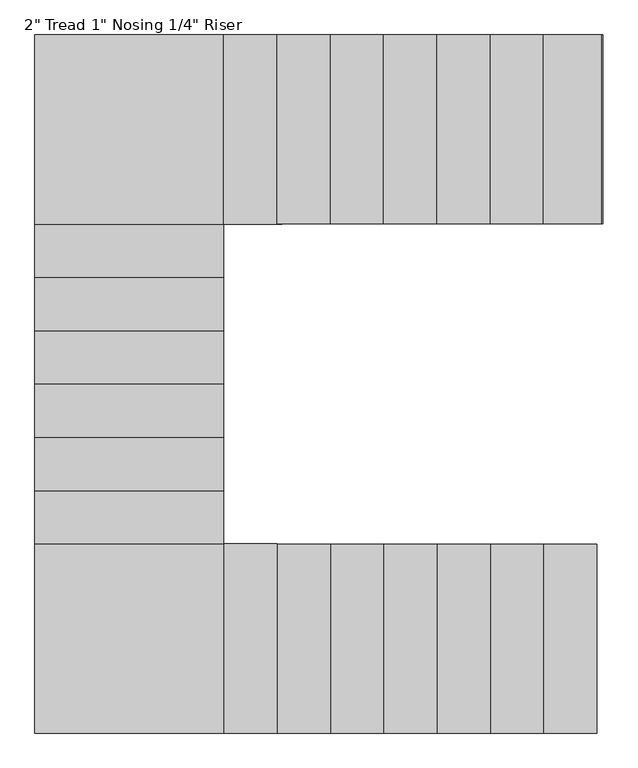
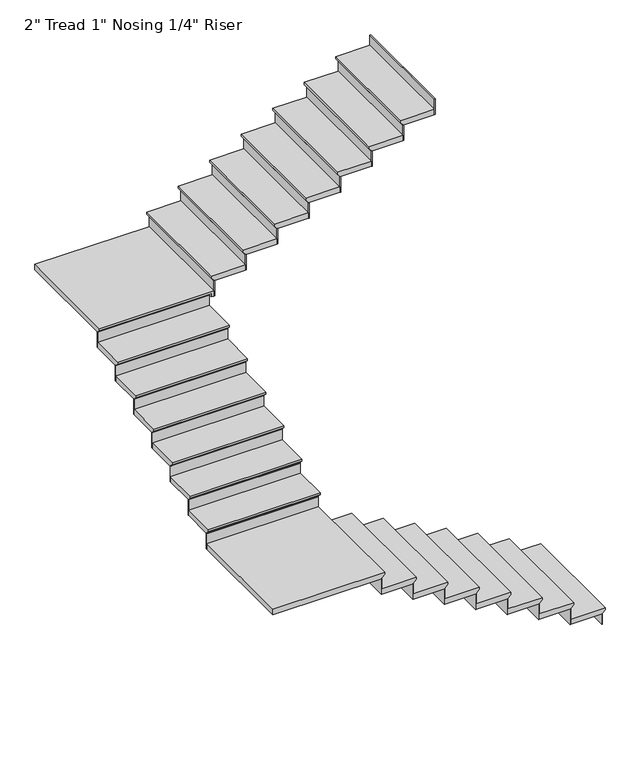
"""IFC4 building model written with IfcOpenShell, lengths in millimetres: stair flight geometry."""

from ifc_helpers import new_model, si_unit, origin, place, context, project, spatial, faceted_brep, source, transform, mapped, element, save


def stair_flight_cb67390f(model_context):
    return source(origin(), model_context, "Body", "Brep", [
        faceted_brep([(14750.242447, -127.8399287, 126.0928571), (14750.242447, -127.8399287, 145.1428571), (14750.242447, -1118.4399287, 145.1428571), (14750.242447, -1118.4399287, 126.0928571), (14724.842447, -127.8399287, 100.6928571), (14724.842447, -1118.4399287, 100.6928571), (14445.442447, -127.8399287, 145.1428571), (14445.442447, -1118.4399287, 145.1428571), (14724.842447, -1118.4399287, 94.3428571), (14445.442447, -1118.4399287, 94.3428571), (14445.442447, -127.8399287, 94.3428571), (14724.842447, -127.8399287, 94.3428571)], [[[0, 1, 2, 3]], [[4, 0, 3, 5]], [[2, 1, 6, 7]], [[8, 9, 10, 11]], [[2, 7, 9, 8, 5, 3]], [[8, 11, 4, 5]], [[6, 1, 0, 4, 11, 10]], [[7, 6, 10, 9]]]),
        faceted_brep([(14724.842447, -127.8399287, 94.3428571), (14724.842447, -127.8399287, 0.0), (14718.492447, -127.8399287, 0.0), (14718.492447, -127.8399287, 94.3428571), (14724.842447, -1118.4399287, 94.3428571), (14718.492447, -1118.4399287, 94.3428571), (14718.492447, -1118.4399287, 0.0), (14724.842447, -1118.4399287, 0.0)], [[[0, 1, 2, 3]], [[4, 5, 6, 7]], [[1, 0, 4, 7]], [[2, 1, 7, 6]], [[3, 2, 6, 5]], [[0, 3, 5, 4]]]),
        faceted_brep([(14445.442447, -127.8399287, 239.4857143), (14445.442447, -127.8399287, 94.3428571), (14439.092447, -127.8399287, 94.3428571), (14439.092447, -127.8399287, 239.4857143), (14445.442447, -1118.4399287, 239.4857143), (14439.092447, -1118.4399287, 239.4857143), (14439.092447, -1118.4399287, 94.3428571), (14445.442447, -1118.4399287, 94.3428571)], [[[0, 1, 2, 3]], [[4, 5, 6, 7]], [[1, 0, 4, 7]], [[2, 1, 7, 6]], [[3, 2, 6, 5]], [[0, 3, 5, 4]]]),
        faceted_brep([(14470.842447, -1118.4399287, 290.2857143), (14470.842447, -127.8399287, 290.2857143), (14166.042447, -127.8399287, 290.2857143), (14166.042447, -1118.4399287, 290.2857143), (14445.442447, -1118.4399287, 239.4857143), (14166.042447, -1118.4399287, 239.4857143), (14166.042447, -127.8399287, 239.4857143), (14445.442447, -127.8399287, 239.4857143), (14445.442447, -1118.4399287, 245.8357143), (14470.842447, -1118.4399287, 271.2357143), (14445.442447, -127.8399287, 245.8357143), (14470.842447, -127.8399287, 271.2357143)], [[[0, 1, 2, 3]], [[4, 5, 6, 7]], [[0, 3, 5, 4, 8, 9]], [[4, 7, 10, 8]], [[2, 1, 11, 10, 7, 6]], [[3, 2, 6, 5]], [[11, 1, 0, 9]], [[10, 11, 9, 8]]]),
        faceted_brep([(14166.042447, -127.8399287, 384.6285714), (14166.042447, -127.8399287, 239.4857143), (14159.692447, -127.8399287, 239.4857143), (14159.692447, -127.8399287, 384.6285714), (14166.042447, -1118.4399287, 384.6285714), (14159.692447, -1118.4399287, 384.6285714), (14159.692447, -1118.4399287, 239.4857143), (14166.042447, -1118.4399287, 239.4857143)], [[[0, 1, 2, 3]], [[4, 5, 6, 7]], [[1, 0, 4, 7]], [[2, 1, 7, 6]], [[3, 2, 6, 5]], [[0, 3, 5, 4]]]),
        faceted_brep([(14191.442447, -1118.4399287, 435.4285714), (14191.442447, -127.8399287, 435.4285714), (13886.642447, -127.8399287, 435.4285714), (13886.642447, -1118.4399287, 435.4285714), (14166.042447, -1118.4399287, 384.6285714), (13886.642447, -1118.4399287, 384.6285714), (13886.642447, -127.8399287, 384.6285714), (14166.042447, -127.8399287, 384.6285714), (14166.042447, -1118.4399287, 390.9785714), (14191.442447, -1118.4399287, 416.3785714), (14166.042447, -127.8399287, 390.9785714), (14191.442447, -127.8399287, 416.3785714)], [[[0, 1, 2, 3]], [[4, 5, 6, 7]], [[0, 3, 5, 4, 8, 9]], [[4, 7, 10, 8]], [[2, 1, 11, 10, 7, 6]], [[3, 2, 6, 5]], [[11, 1, 0, 9]], [[10, 11, 9, 8]]]),
        faceted_brep([(13886.642447, -127.8399287, 529.7714286), (13886.642447, -127.8399287, 384.6285714), (13880.292447, -127.8399287, 384.6285714), (13880.292447, -127.8399287, 529.7714286), (13886.642447, -1118.4399287, 529.7714286), (13880.292447, -1118.4399287, 529.7714286), (13880.292447, -1118.4399287, 384.6285714), (13886.642447, -1118.4399287, 384.6285714)], [[[0, 1, 2, 3]], [[4, 5, 6, 7]], [[1, 0, 4, 7]], [[2, 1, 7, 6]], [[3, 2, 6, 5]], [[0, 3, 5, 4]]]),
        faceted_brep([(13912.042447, -1118.4399287, 580.5714286), (13912.042447, -127.8399287, 580.5714286), (13607.242447, -127.8399287, 580.5714286), (13607.242447, -1118.4399287, 580.5714286), (13886.642447, -1118.4399287, 529.7714286), (13607.242447, -1118.4399287, 529.7714286), (13607.242447, -127.8399287, 529.7714286), (13886.642447, -127.8399287, 529.7714286), (13886.642447, -1118.4399287, 536.1214286), (13912.042447, -1118.4399287, 561.5214286), (13886.642447, -127.8399287, 536.1214286), (13912.042447, -127.8399287, 561.5214286)], [[[0, 1, 2, 3]], [[4, 5, 6, 7]], [[0, 3, 5, 4, 8, 9]], [[4, 7, 10, 8]], [[2, 1, 11, 10, 7, 6]], [[3, 2, 6, 5]], [[11, 1, 0, 9]], [[10, 11, 9, 8]]]),
        faceted_brep([(13607.242447, -127.8399287, 674.9142857), (13607.242447, -127.8399287, 529.7714286), (13600.892447, -127.8399287, 529.7714286), (13600.892447, -127.8399287, 674.9142857), (13607.242447, -1118.4399287, 674.9142857), (13600.892447, -1118.4399287, 674.9142857), (13600.892447, -1118.4399287, 529.7714286), (13607.242447, -1118.4399287, 529.7714286)], [[[0, 1, 2, 3]], [[4, 5, 6, 7]], [[1, 0, 4, 7]], [[2, 1, 7, 6]], [[3, 2, 6, 5]], [[0, 3, 5, 4]]]),
        faceted_brep([(13632.642447, -1118.4399287, 725.7142857), (13632.642447, -127.8399287, 725.7142857), (13327.842447, -127.8399287, 725.7142857), (13327.842447, -1118.4399287, 725.7142857), (13607.242447, -1118.4399287, 674.9142857), (13327.842447, -1118.4399287, 674.9142857), (13327.842447, -127.8399287, 674.9142857), (13607.242447, -127.8399287, 674.9142857), (13607.242447, -1118.4399287, 681.2642857), (13632.642447, -1118.4399287, 706.6642857), (13607.242447, -127.8399287, 681.2642857), (13632.642447, -127.8399287, 706.6642857)], [[[0, 1, 2, 3]], [[4, 5, 6, 7]], [[0, 3, 5, 4, 8, 9]], [[4, 7, 10, 8]], [[2, 1, 11, 10, 7, 6]], [[3, 2, 6, 5]], [[11, 1, 0, 9]], [[10, 11, 9, 8]]]),
        faceted_brep([(13327.842447, -127.8399287, 820.0571429), (13327.842447, -127.8399287, 674.9142857), (13321.492447, -127.8399287, 674.9142857), (13321.492447, -127.8399287, 820.0571429), (13327.842447, -1118.4399287, 820.0571429), (13321.492447, -1118.4399287, 820.0571429), (13321.492447, -1118.4399287, 674.9142857), (13327.842447, -1118.4399287, 674.9142857)], [[[0, 1, 2, 3]], [[4, 5, 6, 7]], [[1, 0, 4, 7]], [[2, 1, 7, 6]], [[3, 2, 6, 5]], [[0, 3, 5, 4]]]),
        faceted_brep([(13353.242447, -1118.4399287, 870.8571429), (13353.242447, -127.8399287, 870.8571429), (13048.442447, -127.8399287, 870.8571429), (13048.442447, -1118.4399287, 870.8571429), (13327.842447, -1118.4399287, 820.0571429), (13048.442447, -1118.4399287, 820.0571429), (13048.442447, -127.8399287, 820.0571429), (13327.842447, -127.8399287, 820.0571429), (13327.842447, -1118.4399287, 826.4071429), (13353.242447, -1118.4399287, 851.8071429), (13327.842447, -127.8399287, 826.4071429), (13353.242447, -127.8399287, 851.8071429)], [[[0, 1, 2, 3]], [[4, 5, 6, 7]], [[0, 3, 5, 4, 8, 9]], [[4, 7, 10, 8]], [[2, 1, 11, 10, 7, 6]], [[3, 2, 6, 5]], [[11, 1, 0, 9]], [[10, 11, 9, 8]]]),
        faceted_brep([(13048.442447, -127.8399287, 965.2), (13048.442447, -127.8399287, 820.0571429), (13042.092447, -127.8399287, 820.0571429), (13042.092447, -127.8399287, 965.2), (13048.442447, -1118.4399287, 965.2), (13042.092447, -1118.4399287, 965.2), (13042.092447, -1118.4399287, 820.0571429), (13048.442447, -1118.4399287, 820.0571429)], [[[0, 1, 2, 3]], [[4, 5, 6, 7]], [[1, 0, 4, 7]], [[2, 1, 7, 6]], [[3, 2, 6, 5]], [[0, 3, 5, 4]]]),
        faceted_brep([(13073.842447, -1118.4399287, 1016.0), (13073.842447, -127.8399287, 1016.0), (12769.042447, -127.8399287, 1016.0), (12769.042447, -1118.4399287, 1016.0), (13048.442447, -1118.4399287, 965.2), (12769.042447, -1118.4399287, 965.2), (12769.042447, -127.8399287, 965.2), (13048.442447, -127.8399287, 965.2), (13048.442447, -1118.4399287, 971.55), (13073.842447, -1118.4399287, 996.95), (13048.442447, -127.8399287, 971.55), (13073.842447, -127.8399287, 996.95)], [[[0, 1, 2, 3]], [[4, 5, 6, 7]], [[0, 3, 5, 4, 8, 9]], [[4, 7, 10, 8]], [[2, 1, 11, 10, 7, 6]], [[3, 2, 6, 5]], [[11, 1, 0, 9]], [[10, 11, 9, 8]]]),
        faceted_brep([(12769.042447, -127.8399287, 1110.3428571), (12769.042447, -127.8399287, 965.2), (12762.692447, -127.8399287, 965.2), (12762.692447, -127.8399287, 1110.3428571), (12769.042447, -1118.4399287, 1110.3428571), (12762.692447, -1118.4399287, 1110.3428571), (12762.692447, -1118.4399287, 965.2), (12769.042447, -1118.4399287, 965.2)], [[[0, 1, 2, 3]], [[4, 5, 6, 7]], [[1, 0, 4, 7]], [[2, 1, 7, 6]], [[3, 2, 6, 5]], [[0, 3, 5, 4]]]),
        faceted_brep([(11803.842447, -102.4399287, 1161.1428571), (11803.842447, -1118.4399287, 1161.1428571), (12794.442447, -1118.4399287, 1161.1428571), (12794.442447, -102.4399287, 1161.1428571), (11803.842447, -1118.4399287, 1110.3428571), (11803.842447, -102.4399287, 1110.3428571), (12794.442447, -102.4399287, 1110.3428571), (12794.442447, -127.8399287, 1110.3428571), (12769.042447, -127.8399287, 1110.3428571), (12769.042447, -1118.4399287, 1110.3428571), (12769.042447, -127.8399287, 1116.6928571), (12769.042447, -1118.4399287, 1116.6928571), (12794.442447, -1118.4399287, 1142.0928571), (12794.442447, -127.8399287, 1142.0928571)], [[[0, 1, 2, 3]], [[4, 5, 6, 7, 8, 9]], [[1, 0, 5, 4]], [[9, 8, 10, 11]], [[3, 2, 12, 13, 7, 6]], [[0, 3, 6, 5]], [[12, 11, 10, 13]], [[2, 1, 4, 9, 11, 12]], [[8, 7, 13, 10]]]),
        faceted_brep([(12794.442447, -102.4399287, 1255.4857143), (12794.442447, -102.4399287, 1110.3428571), (12794.442447, -96.0899287, 1110.3428571), (12794.442447, -96.0899287, 1255.4857143), (11803.842447, -102.4399287, 1255.4857143), (11803.842447, -96.0899287, 1255.4857143), (11803.842447, -96.0899287, 1110.3428571), (11803.842447, -102.4399287, 1110.3428571)], [[[0, 1, 2, 3]], [[4, 5, 6, 7]], [[1, 0, 4, 7]], [[2, 1, 7, 6]], [[3, 2, 6, 5]], [[0, 3, 5, 4]]]),
        faceted_brep([(11803.842447, -127.8399287, 1306.2857143), (12794.442447, -127.8399287, 1306.2857143), (12794.442447, 176.9600713, 1306.2857143), (11803.842447, 176.9600713, 1306.2857143), (11803.842447, -102.4399287, 1255.4857143), (11803.842447, 176.9600713, 1255.4857143), (12794.442447, 176.9600713, 1255.4857143), (12794.442447, -102.4399287, 1255.4857143), (11803.842447, -102.4399287, 1261.8357143), (11803.842447, -127.8399287, 1287.2357143), (12794.442447, -102.4399287, 1261.8357143), (12794.442447, -127.8399287, 1287.2357143)], [[[0, 1, 2, 3]], [[4, 5, 6, 7]], [[0, 3, 5, 4, 8, 9]], [[4, 7, 10, 8]], [[2, 1, 11, 10, 7, 6]], [[3, 2, 6, 5]], [[11, 1, 0, 9]], [[10, 11, 9, 8]]]),
        faceted_brep([(12794.442447, 176.9600713, 1400.6285714), (12794.442447, 176.9600713, 1255.4857143), (12794.442447, 183.3100713, 1255.4857143), (12794.442447, 183.3100713, 1400.6285714), (11803.842447, 176.9600713, 1400.6285714), (11803.842447, 183.3100713, 1400.6285714), (11803.842447, 183.3100713, 1255.4857143), (11803.842447, 176.9600713, 1255.4857143)], [[[0, 1, 2, 3]], [[4, 5, 6, 7]], [[1, 0, 4, 7]], [[2, 1, 7, 6]], [[3, 2, 6, 5]], [[0, 3, 5, 4]]]),
        faceted_brep([(11803.842447, 151.5600713, 1451.4285714), (12794.442447, 151.5600713, 1451.4285714), (12794.442447, 456.3600713, 1451.4285714), (11803.842447, 456.3600713, 1451.4285714), (11803.842447, 176.9600713, 1400.6285714), (11803.842447, 456.3600713, 1400.6285714), (12794.442447, 456.3600713, 1400.6285714), (12794.442447, 176.9600713, 1400.6285714), (11803.842447, 176.9600713, 1406.9785714), (11803.842447, 151.5600713, 1432.3785714), (12794.442447, 176.9600713, 1406.9785714), (12794.442447, 151.5600713, 1432.3785714)], [[[0, 1, 2, 3]], [[4, 5, 6, 7]], [[0, 3, 5, 4, 8, 9]], [[4, 7, 10, 8]], [[2, 1, 11, 10, 7, 6]], [[3, 2, 6, 5]], [[11, 1, 0, 9]], [[10, 11, 9, 8]]]),
        faceted_brep([(12794.442447, 456.3600713, 1545.7714286), (12794.442447, 456.3600713, 1400.6285714), (12794.442447, 462.7100713, 1400.6285714), (12794.442447, 462.7100713, 1545.7714286), (11803.842447, 456.3600713, 1545.7714286), (11803.842447, 462.7100713, 1545.7714286), (11803.842447, 462.7100713, 1400.6285714), (11803.842447, 456.3600713, 1400.6285714)], [[[0, 1, 2, 3]], [[4, 5, 6, 7]], [[1, 0, 4, 7]], [[2, 1, 7, 6]], [[3, 2, 6, 5]], [[0, 3, 5, 4]]]),
        faceted_brep([(11803.842447, 430.9600713, 1596.5714286), (12794.442447, 430.9600713, 1596.5714286), (12794.442447, 735.7600713, 1596.5714286), (11803.842447, 735.7600713, 1596.5714286), (11803.842447, 456.3600713, 1545.7714286), (11803.842447, 735.7600713, 1545.7714286), (12794.442447, 735.7600713, 1545.7714286), (12794.442447, 456.3600713, 1545.7714286), (11803.842447, 456.3600713, 1552.1214286), (11803.842447, 430.9600713, 1577.5214286), (12794.442447, 456.3600713, 1552.1214286), (12794.442447, 430.9600713, 1577.5214286)], [[[0, 1, 2, 3]], [[4, 5, 6, 7]], [[0, 3, 5, 4, 8, 9]], [[4, 7, 10, 8]], [[2, 1, 11, 10, 7, 6]], [[3, 2, 6, 5]], [[11, 1, 0, 9]], [[10, 11, 9, 8]]]),
        faceted_brep([(12794.442447, 735.7600713, 1690.9142857), (12794.442447, 735.7600713, 1545.7714286), (12794.442447, 742.1100713, 1545.7714286), (12794.442447, 742.1100713, 1690.9142857), (11803.842447, 735.7600713, 1690.9142857), (11803.842447, 742.1100713, 1690.9142857), (11803.842447, 742.1100713, 1545.7714286), (11803.842447, 735.7600713, 1545.7714286)], [[[0, 1, 2, 3]], [[4, 5, 6, 7]], [[1, 0, 4, 7]], [[2, 1, 7, 6]], [[3, 2, 6, 5]], [[0, 3, 5, 4]]]),
        faceted_brep([(11803.842447, 710.3600713, 1741.7142857), (12794.442447, 710.3600713, 1741.7142857), (12794.442447, 1015.1600713, 1741.7142857), (11803.842447, 1015.1600713, 1741.7142857), (11803.842447, 735.7600713, 1690.9142857), (11803.842447, 1015.1600713, 1690.9142857), (12794.442447, 1015.1600713, 1690.9142857), (12794.442447, 735.7600713, 1690.9142857), (11803.842447, 735.7600713, 1697.2642857), (11803.842447, 710.3600713, 1722.6642857), (12794.442447, 735.7600713, 1697.2642857), (12794.442447, 710.3600713, 1722.6642857)], [[[0, 1, 2, 3]], [[4, 5, 6, 7]], [[0, 3, 5, 4, 8, 9]], [[4, 7, 10, 8]], [[2, 1, 11, 10, 7, 6]], [[3, 2, 6, 5]], [[11, 1, 0, 9]], [[10, 11, 9, 8]]]),
        faceted_brep([(12794.442447, 1015.1600713, 1836.0571429), (12794.442447, 1015.1600713, 1690.9142857), (12794.442447, 1021.5100713, 1690.9142857), (12794.442447, 1021.5100713, 1836.0571429), (11803.842447, 1015.1600713, 1836.0571429), (11803.842447, 1021.5100713, 1836.0571429), (11803.842447, 1021.5100713, 1690.9142857), (11803.842447, 1015.1600713, 1690.9142857)], [[[0, 1, 2, 3]], [[4, 5, 6, 7]], [[1, 0, 4, 7]], [[2, 1, 7, 6]], [[3, 2, 6, 5]], [[0, 3, 5, 4]]]),
        faceted_brep([(11803.842447, 989.7600713, 1886.8571429), (12794.442447, 989.7600713, 1886.8571429), (12794.442447, 1294.5600713, 1886.8571429), (11803.842447, 1294.5600713, 1886.8571429), (11803.842447, 1015.1600713, 1836.0571429), (11803.842447, 1294.5600713, 1836.0571429), (12794.442447, 1294.5600713, 1836.0571429), (12794.442447, 1015.1600713, 1836.0571429), (11803.842447, 1015.1600713, 1842.4071429), (11803.842447, 989.7600713, 1867.8071429), (12794.442447, 1015.1600713, 1842.4071429), (12794.442447, 989.7600713, 1867.8071429)], [[[0, 1, 2, 3]], [[4, 5, 6, 7]], [[0, 3, 5, 4, 8, 9]], [[4, 7, 10, 8]], [[2, 1, 11, 10, 7, 6]], [[3, 2, 6, 5]], [[11, 1, 0, 9]], [[10, 11, 9, 8]]]),
        faceted_brep([(12794.442447, 1294.5600713, 1981.2), (12794.442447, 1294.5600713, 1836.0571429), (12794.442447, 1300.9100713, 1836.0571429), (12794.442447, 1300.9100713, 1981.2), (11803.842447, 1294.5600713, 1981.2), (11803.842447, 1300.9100713, 1981.2), (11803.842447, 1300.9100713, 1836.0571429), (11803.842447, 1294.5600713, 1836.0571429)], [[[0, 1, 2, 3]], [[4, 5, 6, 7]], [[1, 0, 4, 7]], [[2, 1, 7, 6]], [[3, 2, 6, 5]], [[0, 3, 5, 4]]]),
        faceted_brep([(11803.842447, 1269.1600713, 2032.0), (12794.442447, 1269.1600713, 2032.0), (12794.442447, 1573.9600713, 2032.0), (11803.842447, 1573.9600713, 2032.0), (11803.842447, 1294.5600713, 1981.2), (11803.842447, 1573.9600713, 1981.2), (12794.442447, 1573.9600713, 1981.2), (12794.442447, 1294.5600713, 1981.2), (11803.842447, 1294.5600713, 1987.55), (11803.842447, 1269.1600713, 2012.95), (12794.442447, 1294.5600713, 1987.55), (12794.442447, 1269.1600713, 2012.95)], [[[0, 1, 2, 3]], [[4, 5, 6, 7]], [[0, 3, 5, 4, 8, 9]], [[4, 7, 10, 8]], [[2, 1, 11, 10, 7, 6]], [[3, 2, 6, 5]], [[11, 1, 0, 9]], [[10, 11, 9, 8]]]),
        faceted_brep([(12794.442447, 1573.9600713, 2126.3428571), (12794.442447, 1573.9600713, 1981.2), (12794.442447, 1580.3100713, 1981.2), (12794.442447, 1580.3100713, 2126.3428571), (11803.842447, 1573.9600713, 2126.3428571), (11803.842447, 1580.3100713, 2126.3428571), (11803.842447, 1580.3100713, 1981.2), (11803.842447, 1573.9600713, 1981.2)], [[[0, 1, 2, 3]], [[4, 5, 6, 7]], [[1, 0, 4, 7]], [[2, 1, 7, 6]], [[3, 2, 6, 5]], [[0, 3, 5, 4]]]),
        faceted_brep([(12819.842447, 2539.1600713, 2177.1428571), (11803.842447, 2539.1600713, 2177.1428571), (11803.842447, 1548.5600713, 2177.1428571), (12819.842447, 1548.5600713, 2177.1428571), (11803.842447, 2539.1600713, 2126.3428571), (12819.842447, 2539.1600713, 2126.3428571), (12819.842447, 1548.5600713, 2126.3428571), (12794.442447, 1548.5600713, 2126.3428571), (12794.442447, 1573.9600713, 2126.3428571), (11803.842447, 1573.9600713, 2126.3428571), (12794.442447, 1573.9600713, 2132.6928571), (11803.842447, 1573.9600713, 2132.6928571), (11803.842447, 1548.5600713, 2158.0928571), (12794.442447, 1548.5600713, 2158.0928571)], [[[0, 1, 2, 3]], [[4, 5, 6, 7, 8, 9]], [[1, 0, 5, 4]], [[9, 8, 10, 11]], [[3, 2, 12, 13, 7, 6]], [[0, 3, 6, 5]], [[12, 11, 10, 13]], [[2, 1, 4, 9, 11, 12]], [[8, 7, 13, 10]]]),
        faceted_brep([(12819.842447, 1548.5600713, 2271.4857143), (12819.842447, 1548.5600713, 2126.3428571), (12826.192447, 1548.5600713, 2126.3428571), (12826.192447, 1548.5600713, 2271.4857143), (12819.842447, 2539.1600713, 2271.4857143), (12826.192447, 2539.1600713, 2271.4857143), (12826.192447, 2539.1600713, 2126.3428571), (12819.842447, 2539.1600713, 2126.3428571)], [[[0, 1, 2, 3]], [[4, 5, 6, 7]], [[1, 0, 4, 7]], [[2, 1, 7, 6]], [[3, 2, 6, 5]], [[0, 3, 5, 4]]]),
        faceted_brep([(12794.442447, 2539.1600713, 2322.2857143), (12794.442447, 1548.5600713, 2322.2857143), (13099.242447, 1548.5600713, 2322.2857143), (13099.242447, 2539.1600713, 2322.2857143), (12819.842447, 2539.1600713, 2271.4857143), (13099.242447, 2539.1600713, 2271.4857143), (13099.242447, 1548.5600713, 2271.4857143), (12819.842447, 1548.5600713, 2271.4857143), (12819.842447, 2539.1600713, 2277.8357143), (12794.442447, 2539.1600713, 2303.2357143), (12819.842447, 1548.5600713, 2277.8357143), (12794.442447, 1548.5600713, 2303.2357143)], [[[0, 1, 2, 3]], [[4, 5, 6, 7]], [[0, 3, 5, 4, 8, 9]], [[4, 7, 10, 8]], [[2, 1, 11, 10, 7, 6]], [[3, 2, 6, 5]], [[11, 1, 0, 9]], [[10, 11, 9, 8]]]),
        faceted_brep([(13099.242447, 1548.5600713, 2416.6285714), (13099.242447, 1548.5600713, 2271.4857143), (13105.592447, 1548.5600713, 2271.4857143), (13105.592447, 1548.5600713, 2416.6285714), (13099.242447, 2539.1600713, 2416.6285714), (13105.592447, 2539.1600713, 2416.6285714), (13105.592447, 2539.1600713, 2271.4857143), (13099.242447, 2539.1600713, 2271.4857143)], [[[0, 1, 2, 3]], [[4, 5, 6, 7]], [[1, 0, 4, 7]], [[2, 1, 7, 6]], [[3, 2, 6, 5]], [[0, 3, 5, 4]]]),
        faceted_brep([(13073.842447, 2539.1600713, 2467.4285714), (13073.842447, 1548.5600713, 2467.4285714), (13378.642447, 1548.5600713, 2467.4285714), (13378.642447, 2539.1600713, 2467.4285714), (13099.242447, 2539.1600713, 2416.6285714), (13378.642447, 2539.1600713, 2416.6285714), (13378.642447, 1548.5600713, 2416.6285714), (13099.242447, 1548.5600713, 2416.6285714), (13099.242447, 2539.1600713, 2422.9785714), (13073.842447, 2539.1600713, 2448.3785714), (13099.242447, 1548.5600713, 2422.9785714), (13073.842447, 1548.5600713, 2448.3785714)], [[[0, 1, 2, 3]], [[4, 5, 6, 7]], [[0, 3, 5, 4, 8, 9]], [[4, 7, 10, 8]], [[2, 1, 11, 10, 7, 6]], [[3, 2, 6, 5]], [[11, 1, 0, 9]], [[10, 11, 9, 8]]]),
        faceted_brep([(13378.642447, 1548.5600713, 2561.7714286), (13378.642447, 1548.5600713, 2416.6285714), (13384.992447, 1548.5600713, 2416.6285714), (13384.992447, 1548.5600713, 2561.7714286), (13378.642447, 2539.1600713, 2561.7714286), (13384.992447, 2539.1600713, 2561.7714286), (13384.992447, 2539.1600713, 2416.6285714), (13378.642447, 2539.1600713, 2416.6285714)], [[[0, 1, 2, 3]], [[4, 5, 6, 7]], [[1, 0, 4, 7]], [[2, 1, 7, 6]], [[3, 2, 6, 5]], [[0, 3, 5, 4]]]),
        faceted_brep([(13353.242447, 2539.1600713, 2612.5714286), (13353.242447, 1548.5600713, 2612.5714286), (13658.042447, 1548.5600713, 2612.5714286), (13658.042447, 2539.1600713, 2612.5714286), (13378.642447, 2539.1600713, 2561.7714286), (13658.042447, 2539.1600713, 2561.7714286), (13658.042447, 1548.5600713, 2561.7714286), (13378.642447, 1548.5600713, 2561.7714286), (13378.642447, 2539.1600713, 2568.1214286), (13353.242447, 2539.1600713, 2593.5214286), (13378.642447, 1548.5600713, 2568.1214286), (13353.242447, 1548.5600713, 2593.5214286)], [[[0, 1, 2, 3]], [[4, 5, 6, 7]], [[0, 3, 5, 4, 8, 9]], [[4, 7, 10, 8]], [[2, 1, 11, 10, 7, 6]], [[3, 2, 6, 5]], [[11, 1, 0, 9]], [[10, 11, 9, 8]]]),
        faceted_brep([(13658.042447, 1548.5600713, 2706.9142857), (13658.042447, 1548.5600713, 2561.7714286), (13664.392447, 1548.5600713, 2561.7714286), (13664.392447, 1548.5600713, 2706.9142857), (13658.042447, 2539.1600713, 2706.9142857), (13664.392447, 2539.1600713, 2706.9142857), (13664.392447, 2539.1600713, 2561.7714286), (13658.042447, 2539.1600713, 2561.7714286)], [[[0, 1, 2, 3]], [[4, 5, 6, 7]], [[1, 0, 4, 7]], [[2, 1, 7, 6]], [[3, 2, 6, 5]], [[0, 3, 5, 4]]]),
        faceted_brep([(13632.642447, 2539.1600713, 2757.7142857), (13632.642447, 1548.5600713, 2757.7142857), (13937.442447, 1548.5600713, 2757.7142857), (13937.442447, 2539.1600713, 2757.7142857), (13658.042447, 2539.1600713, 2706.9142857), (13937.442447, 2539.1600713, 2706.9142857), (13937.442447, 1548.5600713, 2706.9142857), (13658.042447, 1548.5600713, 2706.9142857), (13658.042447, 2539.1600713, 2713.2642857), (13632.642447, 2539.1600713, 2738.6642857), (13658.042447, 1548.5600713, 2713.2642857), (13632.642447, 1548.5600713, 2738.6642857)], [[[0, 1, 2, 3]], [[4, 5, 6, 7]], [[0, 3, 5, 4, 8, 9]], [[4, 7, 10, 8]], [[2, 1, 11, 10, 7, 6]], [[3, 2, 6, 5]], [[11, 1, 0, 9]], [[10, 11, 9, 8]]]),
        faceted_brep([(13937.442447, 1548.5600713, 2852.0571429), (13937.442447, 1548.5600713, 2706.9142857), (13943.792447, 1548.5600713, 2706.9142857), (13943.792447, 1548.5600713, 2852.0571429), (13937.442447, 2539.1600713, 2852.0571429), (13943.792447, 2539.1600713, 2852.0571429), (13943.792447, 2539.1600713, 2706.9142857), (13937.442447, 2539.1600713, 2706.9142857)], [[[0, 1, 2, 3]], [[4, 5, 6, 7]], [[1, 0, 4, 7]], [[2, 1, 7, 6]], [[3, 2, 6, 5]], [[0, 3, 5, 4]]]),
        faceted_brep([(13912.042447, 2539.1600713, 2902.8571429), (13912.042447, 1548.5600713, 2902.8571429), (14216.842447, 1548.5600713, 2902.8571429), (14216.842447, 2539.1600713, 2902.8571429), (13937.442447, 2539.1600713, 2852.0571429), (14216.842447, 2539.1600713, 2852.0571429), (14216.842447, 1548.5600713, 2852.0571429), (13937.442447, 1548.5600713, 2852.0571429), (13937.442447, 2539.1600713, 2858.4071429), (13912.042447, 2539.1600713, 2883.8071429), (13937.442447, 1548.5600713, 2858.4071429), (13912.042447, 1548.5600713, 2883.8071429)], [[[0, 1, 2, 3]], [[4, 5, 6, 7]], [[0, 3, 5, 4, 8, 9]], [[4, 7, 10, 8]], [[2, 1, 11, 10, 7, 6]], [[3, 2, 6, 5]], [[11, 1, 0, 9]], [[10, 11, 9, 8]]]),
        faceted_brep([(14216.842447, 1548.5600713, 2997.2), (14216.842447, 1548.5600713, 2852.0571429), (14223.192447, 1548.5600713, 2852.0571429), (14223.192447, 1548.5600713, 2997.2), (14216.842447, 2539.1600713, 2997.2), (14223.192447, 2539.1600713, 2997.2), (14223.192447, 2539.1600713, 2852.0571429), (14216.842447, 2539.1600713, 2852.0571429)], [[[0, 1, 2, 3]], [[4, 5, 6, 7]], [[1, 0, 4, 7]], [[2, 1, 7, 6]], [[3, 2, 6, 5]], [[0, 3, 5, 4]]]),
        faceted_brep([(14191.442447, 2539.1600713, 3048.0), (14191.442447, 1548.5600713, 3048.0), (14496.242447, 1548.5600713, 3048.0), (14496.242447, 2539.1600713, 3048.0), (14216.842447, 2539.1600713, 2997.2), (14496.242447, 2539.1600713, 2997.2), (14496.242447, 1548.5600713, 2997.2), (14216.842447, 1548.5600713, 2997.2), (14216.842447, 2539.1600713, 3003.55), (14191.442447, 2539.1600713, 3028.95), (14216.842447, 1548.5600713, 3003.55), (14191.442447, 1548.5600713, 3028.95)], [[[0, 1, 2, 3]], [[4, 5, 6, 7]], [[0, 3, 5, 4, 8, 9]], [[4, 7, 10, 8]], [[2, 1, 11, 10, 7, 6]], [[3, 2, 6, 5]], [[11, 1, 0, 9]], [[10, 11, 9, 8]]]),
        faceted_brep([(14496.242447, 1548.5600713, 3142.3428571), (14496.242447, 1548.5600713, 2997.2), (14502.592447, 1548.5600713, 2997.2), (14502.592447, 1548.5600713, 3142.3428571), (14496.242447, 2539.1600713, 3142.3428571), (14502.592447, 2539.1600713, 3142.3428571), (14502.592447, 2539.1600713, 2997.2), (14496.242447, 2539.1600713, 2997.2)], [[[0, 1, 2, 3]], [[4, 5, 6, 7]], [[1, 0, 4, 7]], [[2, 1, 7, 6]], [[3, 2, 6, 5]], [[0, 3, 5, 4]]]),
        faceted_brep([(14775.642447, 1548.5600713, 3287.4857143), (14775.642447, 1548.5600713, 3142.3428571), (14781.992447, 1548.5600713, 3142.3428571), (14781.992447, 1548.5600713, 3287.4857143), (14775.642447, 2539.1600713, 3287.4857143), (14781.992447, 2539.1600713, 3287.4857143), (14781.992447, 2539.1600713, 3142.3428571), (14775.642447, 2539.1600713, 3142.3428571)], [[[0, 1, 2, 3]], [[4, 5, 6, 7]], [[1, 0, 4, 7]], [[2, 1, 7, 6]], [[3, 2, 6, 5]], [[0, 3, 5, 4]]]),
        faceted_brep([(14470.842447, 2539.1600713, 3193.1428571), (14470.842447, 1548.5600713, 3193.1428571), (14775.642447, 1548.5600713, 3193.1428571), (14775.642447, 2539.1600713, 3193.1428571), (14496.242447, 2539.1600713, 3142.3428571), (14775.642447, 2539.1600713, 3142.3428571), (14775.642447, 1548.5600713, 3142.3428571), (14496.242447, 1548.5600713, 3142.3428571), (14496.242447, 2539.1600713, 3148.6928571), (14470.842447, 2539.1600713, 3174.0928571), (14496.242447, 1548.5600713, 3148.6928571), (14470.842447, 1548.5600713, 3174.0928571)], [[[0, 1, 2, 3]], [[4, 5, 6, 7]], [[0, 3, 5, 4, 8, 9]], [[4, 7, 10, 8]], [[2, 1, 11, 10, 7, 6]], [[3, 2, 6, 5]], [[11, 1, 0, 9]], [[10, 11, 9, 8]]]),
    ])


if __name__ == "__main__":
    model = new_model("IFC4")
    model_context = context("Model", 3, world=origin())
    ifc_project = project(units=[si_unit("LENGTHUNIT", "METRE", prefix="MILLI")], contexts=[model_context])
    site = spatial("IfcSite", under=ifc_project)
    building = spatial("IfcBuilding", under=site)
    placement = place(None, origin())
    stair_flight_shape = stair_flight_cb67390f(model_context)
    element("IfcStairFlight", 1, ObjectType="2\" Tread 1\" Nosing 1/4\" Riser", at=placement, inside=building, context=model_context, shape_type="MappedRepresentation", body=[
        mapped(stair_flight_shape, transform((0.0, 0.0, 0.0), x_axis=(1.0, 0.0, 0.0), y_axis=(0.0, 1.0, 0.0), z_axis=(0.0, 0.0, 1.0))),
    ])
    save(model, "model.ifc")
